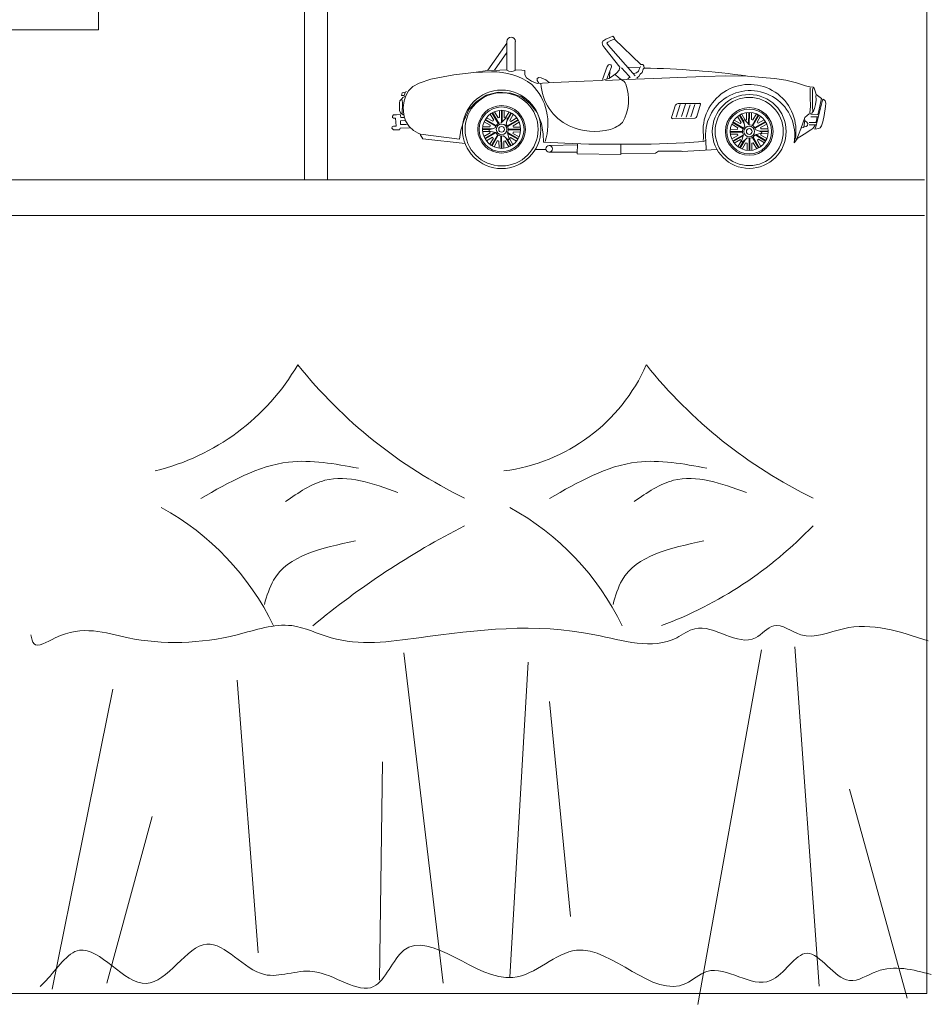
# Model space of a CAD drawing. Units: inches. Extents: x -17 to 1735, y -531 to 60.
# Tile 17 of 27: x 1734.789 to 1734.82808, y -150.26502 to -150.22283. Entities that reach past the tile are written whole.
import ezdxf

# ---------------------------------------------------------------- set-up
doc = ezdxf.new("R2010")
doc.units = ezdxf.units.IN
doc.header["$MEASUREMENT"] = 0
doc.layers.add('A-FURN', color=242, linetype='Continuous', lineweight=18, true_color=0xcd2027)

# ---------------------------------------------------------------- blocks, each defined once
blk = doc.blocks.new('childrens_room_2')
for p, q in [((74.0483, 55.5336), (74.0483, 52.9336)), ((73.1463, 53.9825), (73.1463, 54.7238)), ((73.3706, 53.8193), (73.3706, 54.1771)), ((73.3956, 53.8193), (73.3956, 54.1771)), ((72.0693, 53.9825), (73.1463, 53.9825)), ((73.6988, 53.9726), (73.6953, 53.9704)), ((73.703, 53.9741), (73.6988, 53.9726)), ((73.7062, 53.9758), (73.703, 53.9741)), ((73.7077, 53.9723), (73.7033, 53.9706)), ((73.7071, 53.9751), (73.7062, 53.9758)), ((73.7086, 53.9727), (73.7071, 53.9751)), ((73.7081, 53.9724), (73.7086, 53.9727)), ((73.7368, 53.9448), (73.7081, 53.9724)), ((73.591, 53.9681), (73.5703, 53.9388)), ((73.591, 53.9699), (73.591, 53.9386)), ((73.6001, 53.9382), (73.6001, 53.9699)), ((73.6953, 53.9704), (73.6946, 53.9686)), ((73.6946, 53.9686), (73.6953, 53.9656)), ((73.6953, 53.9656), (73.6975, 53.9626)), ((73.6975, 53.9626), (73.7141, 53.9421)), ((73.7007, 53.9693), (73.6998, 53.968)), ((73.6998, 53.968), (73.7003, 53.9672)), ((73.7003, 53.9672), (73.7041, 53.9626)), ((73.7033, 53.9706), (73.7007, 53.9693)), ((73.7041, 53.9626), (73.7282, 53.9356)), ((73.591, 53.9579), (73.5774, 53.9387)), ((73.7001, 53.9427), (73.6952, 53.9284)), ((73.6998, 53.9292), (73.7047, 53.9422)), ((73.7015, 53.9444), (73.7001, 53.9427)), ((73.7026, 53.945), (73.7015, 53.9444)), ((73.704, 53.9447), (73.7026, 53.945)), ((73.7046, 53.944), (73.704, 53.9447)), ((73.7047, 53.9432), (73.7046, 53.944)), ((73.7047, 53.9422), (73.7047, 53.9432)), ((73.7141, 53.9421), (73.7132, 53.9386)), ((73.7157, 53.9412), (73.7237, 53.9327)), ((73.7356, 53.9413), (73.723, 53.942)), ((73.7342, 53.9377), (73.7354, 53.9405)), ((73.7354, 53.9405), (73.7365, 53.9428)), ((73.7388, 53.9448), (73.7368, 53.9448)), ((73.7402, 53.9433), (73.7388, 53.9448)), ((73.7395, 53.9398), (73.7403, 53.9409)), ((73.7403, 53.9409), (73.7402, 53.9433)), ((73.5333, 53.9338), (73.5083, 53.9288)), ((73.5551, 53.9362), (73.5333, 53.9338)), ((73.57, 53.9382), (73.5551, 53.9362)), ((73.5742, 53.9368), (73.5551, 53.9362)), ((73.5831, 53.9387), (73.57, 53.9382)), ((73.591, 53.9389), (73.5831, 53.9387)), ((73.6073, 53.9386), (73.6001, 53.9389)), ((73.6106, 53.9383), (73.6073, 53.9386)), ((73.6106, 53.9383), (73.6104, 53.9335)), ((73.6104, 53.9335), (73.6123, 53.9305)), ((73.6123, 53.9305), (73.6176, 53.9268)), ((73.6256, 53.9307), (73.6238, 53.9298)), ((73.6238, 53.9298), (73.6238, 53.9275)), ((73.6282, 53.9303), (73.6256, 53.9307)), ((73.6335, 53.9281), (73.6282, 53.9303)), ((73.7019, 53.9297), (73.6944, 53.9276)), ((73.7058, 53.9323), (73.7019, 53.9297)), ((73.7027, 53.9308), (73.703, 53.9372)), ((73.7102, 53.9353), (73.7058, 53.9323)), ((73.7093, 53.9335), (73.7124, 53.9308)), ((73.7132, 53.9386), (73.7102, 53.9353)), ((73.7124, 53.9308), (73.7169, 53.9275)), ((73.751, 53.9297), (73.7208, 53.9284)), ((73.7238, 53.9304), (73.7228, 53.9292)), ((73.7237, 53.9327), (73.7252, 53.9309)), ((73.7252, 53.9309), (73.7238, 53.9304)), ((73.7282, 53.9356), (73.7307, 53.9327)), ((73.7292, 53.935), (73.7319, 53.9358)), ((73.7319, 53.9358), (73.7342, 53.9377)), ((73.7325, 53.93), (73.7335, 53.931)), ((73.7335, 53.931), (73.7345, 53.9319)), ((73.7345, 53.9319), (73.7362, 53.9343)), ((73.7362, 53.9343), (73.7383, 53.9363)), ((73.7383, 53.9363), (73.7395, 53.9398)), ((73.7769, 53.9307), (73.751, 53.9297)), ((73.8064, 53.932), (73.7769, 53.9307)), ((73.8292, 53.9324), (73.8064, 53.932)), ((73.853, 53.9323), (73.8292, 53.9324)), ((73.853, 53.9323), (73.8495, 53.9328)), ((73.8688, 53.9308), (73.853, 53.9323)), ((73.8822, 53.9295), (73.8688, 53.9308)), ((73.8945, 53.9278), (73.8822, 53.9295)), ((73.4884, 53.9208), (73.484, 53.9163)), ((73.4955, 53.9247), (73.4884, 53.9208)), ((73.5083, 53.9288), (73.4955, 53.9247)), ((73.6176, 53.9268), (73.6239, 53.9242)), ((73.6238, 53.9275), (73.6258, 53.9244)), ((73.6416, 53.9252), (73.6239, 53.9242)), ((73.6369, 53.9253), (73.6335, 53.9281)), ((73.6751, 53.9268), (73.6416, 53.9252)), ((73.6944, 53.9276), (73.6751, 53.9268)), ((73.7208, 53.9284), (73.6983, 53.9276)), ((73.9063, 53.9251), (73.8945, 53.9278)), ((73.9161, 53.9218), (73.9063, 53.9251)), ((73.9208, 53.9204), (73.9161, 53.9218)), ((73.9244, 53.9201), (73.9208, 53.9204)), ((73.9212, 53.9195), (73.9213, 53.9094)), ((73.924, 53.919), (73.9237, 53.9167)), ((73.9255, 53.9192), (73.9244, 53.9201)), ((73.9269, 53.9149), (73.9255, 53.9192)), ((73.4764, 53.9111), (73.4768, 53.9141)), ((73.479, 53.9111), (73.4764, 53.9111)), ((73.4766, 53.9075), (73.4778, 53.909)), ((73.4768, 53.9141), (73.4788, 53.9144)), ((73.4778, 53.909), (73.4799, 53.9102)), ((73.4788, 53.9144), (73.4803, 53.9148)), ((73.481, 53.9107), (73.4792, 53.9053)), ((73.4794, 53.9114), (73.4803, 53.9147)), ((73.4803, 53.9148), (73.4818, 53.9155)), ((73.484, 53.9163), (73.481, 53.9107)), ((73.5576, 53.9041), (73.5685, 53.9114)), ((73.5685, 53.9114), (73.5814, 53.9147)), ((73.5814, 53.9147), (73.5954, 53.9137)), ((73.5954, 53.9137), (73.6067, 53.9096)), ((73.6067, 53.9096), (73.6154, 53.9028)), ((73.9213, 53.9094), (73.9215, 53.8992)), ((73.9237, 53.9167), (73.9237, 53.8989)), ((73.9275, 53.9121), (73.9269, 53.9149)), ((73.9273, 53.911), (73.9275, 53.9062)), ((73.9336, 53.9077), (73.9275, 53.9121)), ((73.9329, 53.9045), (73.9336, 53.9079)), ((73.9336, 53.9079), (73.9336, 53.9077)), ((73.474, 53.8949), (73.4742, 53.9033)), ((73.4742, 53.9033), (73.4745, 53.9054)), ((73.4745, 53.9054), (73.4757, 53.9067)), ((73.4757, 53.9067), (73.4766, 53.9075)), ((73.4772, 53.9029), (73.4769, 53.9064)), ((73.4769, 53.8917), (73.4772, 53.9029)), ((73.4792, 53.9053), (73.4779, 53.898)), ((73.4779, 53.898), (73.4787, 53.89)), ((73.5499, 53.8961), (73.5576, 53.9041)), ((73.6154, 53.9028), (73.6239, 53.8928)), ((73.7705, 53.8884), (73.7747, 53.9011)), ((73.7753, 53.8877), (73.7795, 53.9012)), ((73.7782, 53.9025), (73.7986, 53.9024)), ((73.7809, 53.8884), (73.7854, 53.9017)), ((73.786, 53.8875), (73.7904, 53.9009)), ((73.7912, 53.8878), (73.7956, 53.9014)), ((73.8018, 53.9016), (73.7977, 53.8882)), ((73.7986, 53.9024), (73.8009, 53.9026)), ((73.9215, 53.8992), (73.9209, 53.8923)), ((73.9237, 53.8989), (73.924, 53.894)), ((73.9258, 53.897), (73.9248, 53.8942)), ((73.9268, 53.9012), (73.9258, 53.897)), ((73.9275, 53.9062), (73.9268, 53.9012)), ((73.9344, 53.9062), (73.9273, 53.877)), ((73.9309, 53.8964), (73.9329, 53.9045)), ((73.9354, 53.9073), (73.9344, 53.9062)), ((73.9354, 53.9073), (73.9365, 53.9066)), ((73.9377, 53.8991), (73.9363, 53.8894)), ((73.9365, 53.9066), (73.9375, 53.9055)), ((73.9375, 53.9055), (73.9382, 53.9028)), ((73.9382, 53.9028), (73.9377, 53.8991)), ((73.4664, 53.8886), (73.4676, 53.89)), ((73.4666, 53.8873), (73.4664, 53.8886)), ((73.4675, 53.8863), (73.4666, 53.8873)), ((73.4696, 53.8863), (73.4675, 53.8863)), ((73.4676, 53.89), (73.4708, 53.8902)), ((73.4704, 53.8777), (73.4696, 53.8863)), ((73.4708, 53.8902), (73.4746, 53.8905)), ((73.475, 53.8921), (73.474, 53.8949)), ((73.4746, 53.8905), (73.4751, 53.8892)), ((73.4758, 53.8916), (73.475, 53.8921)), ((73.4751, 53.8892), (73.4755, 53.8871)), ((73.4755, 53.8871), (73.4787, 53.8871)), ((73.4778, 53.8905), (73.4758, 53.8916)), ((73.4781, 53.8898), (73.4778, 53.8905)), ((73.4787, 53.89), (73.4804, 53.8836)), ((73.5441, 53.8834), (73.5499, 53.8961)), ((73.5755, 53.8832), (73.5689, 53.887)), ((73.5767, 53.8843), (73.5728, 53.8909)), ((73.5815, 53.8806), (73.5747, 53.8921)), ((73.5822, 53.8809), (73.5753, 53.8925)), ((73.5813, 53.8868), (73.5774, 53.8935)), ((73.5828, 53.8872), (73.5828, 53.8948)), ((73.5851, 53.8816), (73.585, 53.895)), ((73.5852, 53.8816), (73.5901, 53.8869)), ((73.5859, 53.8823), (73.5857, 53.895)), ((73.5881, 53.8871), (73.588, 53.8948)), ((73.5896, 53.8867), (73.5933, 53.8933)), ((73.5901, 53.8869), (73.5915, 53.8863)), ((73.5915, 53.8863), (73.5901, 53.8797)), ((73.5907, 53.8826), (73.596, 53.8919)), ((73.5912, 53.885), (73.5954, 53.8923)), ((73.5941, 53.884), (73.5979, 53.8906)), ((73.5952, 53.8828), (73.6017, 53.8867)), ((73.6239, 53.8928), (73.6285, 53.8805)), ((73.7957, 53.8865), (73.7716, 53.8858)), ((73.8459, 53.8816), (73.8421, 53.8883)), ((73.8493, 53.8802), (73.844, 53.8896)), ((73.8488, 53.8827), (73.8446, 53.89)), ((73.8504, 53.8843), (73.8467, 53.891)), ((73.8519, 53.8848), (73.852, 53.8924)), ((73.8541, 53.8799), (73.8543, 53.8926)), ((73.8549, 53.8792), (73.855, 53.8926)), ((73.8572, 53.8849), (73.8573, 53.8925)), ((73.8579, 53.8786), (73.8647, 53.8902)), ((73.8585, 53.8782), (73.8653, 53.8898)), ((73.8587, 53.8845), (73.8626, 53.8911)), ((73.8633, 53.882), (73.8672, 53.8885)), ((73.9153, 53.8871), (73.9132, 53.8811)), ((73.9179, 53.8893), (73.9153, 53.8871)), ((73.9202, 53.8912), (73.9179, 53.8893)), ((73.9229, 53.892), (73.9202, 53.8912)), ((73.9299, 53.8902), (73.922, 53.8903)), ((73.9295, 53.8878), (73.922, 53.8878)), ((73.9242, 53.8932), (73.9229, 53.892)), ((73.9248, 53.8942), (73.9242, 53.8932)), ((73.9281, 53.8841), (73.9289, 53.8878)), ((73.9295, 53.8902), (73.9309, 53.8964)), ((73.9363, 53.8894), (73.9348, 53.8823)), ((73.4658, 53.8755), (73.466, 53.877)), ((73.466, 53.877), (73.4676, 53.8776)), ((73.4676, 53.8776), (73.4704, 53.8777)), ((73.4849, 53.8758), (73.4749, 53.8755)), ((73.4751, 53.8837), (73.48, 53.8839)), ((73.4752, 53.8796), (73.4751, 53.8837)), ((73.4816, 53.8794), (73.4752, 53.8796)), ((73.4804, 53.8836), (73.4846, 53.8775)), ((73.4846, 53.8775), (73.4894, 53.873)), ((73.5409, 53.8735), (73.5441, 53.8834)), ((73.5724, 53.8772), (73.5647, 53.8771)), ((73.5728, 53.8787), (73.5662, 53.8825)), ((73.5789, 53.8779), (73.5672, 53.8845)), ((73.5793, 53.8785), (73.5676, 53.8851)), ((73.5716, 53.8738), (73.5781, 53.8759)), ((73.5914, 53.878), (73.603, 53.8848)), ((73.5918, 53.8773), (73.6034, 53.8842)), ((73.5977, 53.8782), (73.6043, 53.8821)), ((73.5981, 53.8767), (73.6057, 53.8767)), ((73.6285, 53.8805), (73.6306, 53.8689)), ((73.8423, 53.8759), (73.8357, 53.8798)), ((73.8482, 53.875), (73.8366, 53.8818)), ((73.8486, 53.8757), (73.837, 53.8825)), ((73.8448, 53.8805), (73.8383, 53.8843)), ((73.8499, 53.8846), (73.8485, 53.884)), ((73.8485, 53.884), (73.8499, 53.8773)), ((73.8548, 53.8792), (73.8499, 53.8846)), ((73.8608, 53.8762), (73.8725, 53.8828)), ((73.8612, 53.8755), (73.8728, 53.8821)), ((73.8645, 53.8809), (73.8712, 53.8846)), ((73.8672, 53.8764), (73.8738, 53.8801)), ((73.9132, 53.8811), (73.911, 53.8747)), ((73.9142, 53.8763), (73.912, 53.8758)), ((73.9144, 53.8765), (73.9142, 53.8763)), ((73.9154, 53.8842), (73.9144, 53.8765)), ((73.9167, 53.8773), (73.9145, 53.8771)), ((73.9151, 53.8845), (73.9154, 53.8842)), ((73.9155, 53.8835), (73.917, 53.8826)), ((73.9183, 53.8785), (73.9167, 53.8773)), ((73.917, 53.8826), (73.9185, 53.8808)), ((73.9185, 53.8808), (73.9183, 53.8785)), ((73.9281, 53.8816), (73.9201, 53.8816)), ((73.9277, 53.8792), (73.9201, 53.8792)), ((73.9242, 53.8753), (73.9261, 53.8781)), ((73.9261, 53.8781), (73.9264, 53.8792)), ((73.9273, 53.877), (73.9262, 53.8744)), ((73.9272, 53.8816), (73.9281, 53.8841)), ((73.9322, 53.8761), (73.9306, 53.8751)), ((73.9335, 53.8781), (73.9322, 53.8761)), ((73.9348, 53.8823), (73.9335, 53.8781)), ((73.4676, 53.8737), (73.4658, 53.8755)), ((73.4698, 53.8737), (73.4676, 53.8737)), ((73.4739, 53.8737), (73.4698, 53.8737)), ((73.4749, 53.8755), (73.4739, 53.8737)), ((73.4894, 53.873), (73.4942, 53.8701)), ((73.4942, 53.8701), (73.4969, 53.8692)), ((73.4995, 53.8641), (73.4965, 53.8688)), ((73.4969, 53.8692), (73.5392, 53.8636)), ((73.5392, 53.8636), (73.5409, 53.8735)), ((73.5752, 53.875), (73.5645, 53.8749)), ((73.5729, 53.8742), (73.5645, 53.8741)), ((73.5723, 53.872), (73.5646, 53.8719)), ((73.5727, 53.8704), (73.566, 53.8665)), ((73.5779, 53.8709), (73.567, 53.8645)), ((73.5789, 53.8706), (73.5674, 53.8638)), ((73.5752, 53.8658), (73.5686, 53.8619)), ((73.5718, 53.8723), (73.5716, 53.8738)), ((73.5789, 53.8707), (73.5718, 53.8723)), ((73.581, 53.8684), (73.5743, 53.8567)), ((73.5816, 53.868), (73.575, 53.8563)), ((73.5845, 53.8671), (73.5846, 53.8536)), ((73.5852, 53.867), (73.5854, 53.8536)), ((73.5924, 53.8628), (73.5873, 53.8674)), ((73.5896, 53.8654), (73.595, 53.8561)), ((73.5915, 53.8707), (73.6032, 53.8641)), ((73.5915, 53.8706), (73.5936, 53.8637)), ((73.5917, 53.8697), (73.6028, 53.8635)), ((73.5924, 53.8736), (73.6059, 53.8737)), ((73.5925, 53.8744), (73.6059, 53.8745)), ((73.5948, 53.8654), (73.6015, 53.8616)), ((73.5975, 53.8699), (73.6042, 53.8662)), ((73.598, 53.8714), (73.6057, 53.8715)), ((73.6306, 53.8689), (73.631, 53.8603)), ((73.8045, 53.8741), (73.8051, 53.8651)), ((73.8051, 53.8651), (73.8048, 53.8622)), ((73.8476, 53.8713), (73.8341, 53.8714)), ((73.8476, 53.872), (73.8342, 53.8721)), ((73.8419, 53.8743), (73.8343, 53.8744)), ((73.842, 53.8691), (73.8343, 53.8691)), ((73.8425, 53.8676), (73.8358, 53.8638)), ((73.8485, 53.8684), (73.8368, 53.8618)), ((73.8483, 53.8674), (73.8372, 53.8611)), ((73.8485, 53.8683), (73.8464, 53.8613)), ((73.8476, 53.8605), (73.8527, 53.865)), ((73.8584, 53.8656), (73.865, 53.854)), ((73.859, 53.866), (73.8657, 53.8543)), ((73.8611, 53.8684), (73.8682, 53.87)), ((73.8611, 53.8683), (73.8726, 53.8615)), ((73.8684, 53.8714), (73.8619, 53.8736)), ((73.8621, 53.8686), (73.873, 53.8621)), ((73.8648, 53.8726), (73.8755, 53.8725)), ((73.8671, 53.8719), (73.8755, 53.8718)), ((73.8674, 53.8681), (73.874, 53.8642)), ((73.8676, 53.8748), (73.8753, 53.8748)), ((73.8677, 53.8696), (73.8754, 53.8695)), ((73.8682, 53.87), (73.8684, 53.8714)), ((73.9085, 53.8682), (73.9057, 53.862)), ((73.9071, 53.8645), (73.9147, 53.8689)), ((73.911, 53.8747), (73.9085, 53.8682)), ((73.9147, 53.8689), (73.9219, 53.8736)), ((73.9219, 53.8736), (73.9242, 53.8753)), ((73.9306, 53.8751), (73.9262, 53.8744)), ((73.5455, 53.859), (73.4995, 53.8641)), ((73.5763, 53.8647), (73.5725, 53.858)), ((73.5808, 53.862), (73.577, 53.8553)), ((73.5823, 53.8615), (73.5824, 53.8538)), ((73.5875, 53.8614), (73.5876, 53.8538)), ((73.5891, 53.8618), (73.593, 53.8552)), ((73.5914, 53.8637), (73.5957, 53.8565)), ((73.5936, 53.8637), (73.5924, 53.8628)), ((73.5937, 53.8643), (73.5975, 53.8577)), ((73.631, 53.8603), (73.6542, 53.8593)), ((73.6369, 53.8567), (73.6678, 53.8573)), ((73.6542, 53.8593), (73.68, 53.8583)), ((73.6676, 53.8477), (73.668, 53.8586)), ((73.68, 53.8583), (73.7124, 53.858)), ((73.7124, 53.858), (73.7479, 53.8581)), ((73.7149, 53.8579), (73.7149, 53.8469)), ((73.7845, 53.8598), (73.7479, 53.8581)), ((73.7845, 53.8598), (73.8046, 53.8611)), ((73.8046, 53.8611), (73.8076, 53.8622)), ((73.8076, 53.8622), (73.8081, 53.8517)), ((73.8452, 53.8631), (73.8385, 53.8593)), ((73.8463, 53.862), (73.8425, 53.8554)), ((73.8486, 53.8614), (73.8443, 53.8541)), ((73.8504, 53.863), (73.845, 53.8538)), ((73.8464, 53.8613), (73.8476, 53.8605)), ((73.8509, 53.8594), (73.847, 53.8528)), ((73.8525, 53.8591), (73.8524, 53.8514)), ((73.8548, 53.8647), (73.8546, 53.8513)), ((73.8555, 53.8647), (73.8554, 53.8513)), ((73.8577, 53.8592), (73.8576, 53.8515)), ((73.8592, 53.8596), (73.863, 53.853)), ((73.8637, 53.8623), (73.8675, 53.8556)), ((73.8648, 53.8635), (73.8714, 53.8596)), ((73.9038, 53.8597), (73.9053, 53.8613)), ((73.9053, 53.8613), (73.9069, 53.8641)), ((73.9069, 53.8641), (73.9071, 53.8645)), ((73.6333, 53.8524), (73.6223, 53.8524)), ((73.6678, 53.8495), (73.6368, 53.8495)), ((73.7149, 53.8469), (73.6676, 53.8477)), ((73.7528, 53.8483), (73.7149, 53.8479)), ((73.7562, 53.8507), (73.7528, 53.8483)), ((73.7811, 53.8506), (73.7562, 53.8507)), ((73.7819, 53.8503), (73.7811, 53.8506)), ((73.7819, 53.8503), (73.8197, 53.8523)), ((73.0463, 53.8193), (74.0458, 53.8193)), ((73.0463, 53.7804), (74.0458, 53.7804)), ((73.8682, 53.3077), (73.7989, 52.9219)), ((73.9045, 53.311), (73.9309, 52.9417)), ((73.4788, 53.3044), (73.5217, 52.945)), ((73.6141, 53.2945), (73.5943, 52.9516)), ((73.1619, 53.2648), (73.0959, 52.9384)), ((73.2972, 53.2747), (73.3203, 52.978)), ((73.6372, 53.2516), (73.6603, 53.0175)), ((73.4557, 53.1857), (73.4524, 52.9483)), ((73.9639, 53.156), (74.0266, 52.9285)), ((73.2048, 53.1263), (73.1553, 52.945)), ((72.0483, 52.9336), (74.0483, 52.9336))]:
    blk.add_line(p, q)
blk.add_lwpolyline([(73.628, 53.9242, 0.277279), (73.6587, 53.8781, 0.17984), (73.7036, 53.8743, 0.128199), (73.7167, 53.8819, 0.227122), (73.7203, 53.9236, 0.200085), (73.7159, 53.9282, 1.871987)], format="xyb")
for centre, radius in [((73.5852, 53.8743), 0.0427), ((73.5852, 53.8743), 0.0398), ((73.8548, 53.872), 0.0402), ((73.8548, 53.872), 0.0371), ((73.5852, 53.8743), 0.0259), ((73.5852, 53.8743), 0.0244), ((73.8548, 53.872), 0.0259), ((73.5852, 53.8743), 0.0207), ((73.8548, 53.872), 0.0244), ((73.8548, 53.872), 0.0207), ((73.5852, 53.8743), 0.00582), ((73.5852, 53.8743), 0.00313), ((73.8548, 53.872), 0.00582), ((73.8548, 53.872), 0.00313), ((73.6369, 53.8531), 0.00358)]:
    blk.add_circle(centre, radius)
for centre, radius, start, end in [((73.5956, 53.9699), 0.00456, 0, 180), ((73.725, 52.9996), 0.9415, 82.1883, 89.069), ((73.5773, 53.8693), 0.0675, 52.7792, 92.6699), ((73.5959, 53.9473), 0.01, 240.6981, 294.7246), ((73.5751, 53.8805), 0.0606, 341.2239, 44.7052), ((73.8551, 53.8726), 0.0506, 349.8147, 178.3468), ((73.8558, 53.8679), 0.0486, 350.3249, 186.7561), ((73.7778, 53.8985), 0.00399, 83.8396, 139.4858), ((73.8008, 53.9016), 0.00104, 1.1933, 81.4781), ((73.5852, 53.8743), 0.0131, 100.363, 107.2977), ((73.5852, 53.8743), 0.0131, 70.363, 77.2977), ((73.772, 53.8875), 0.00178, 149.6689, 255.8381), ((73.7942, 53.8902), 0.00408, 292.5869, 329.881), ((73.5852, 53.8743), 0.0131, 160.363, 167.2977), ((73.5852, 53.8743), 0.0131, 130.363, 137.2977), ((73.5852, 53.8743), 0.00727, 89.6688, 167.3416), ((73.5852, 53.8743), 0.00727, 329.6688, 47.3416), ((73.5852, 53.8743), 0.0131, 40.363, 47.2977), ((73.5852, 53.8743), 0.0131, 10.363, 17.2977), ((73.8548, 53.872), 0.0131, 162.7023, 169.637), ((73.8548, 53.872), 0.0131, 132.7023, 139.637), ((73.8548, 53.872), 0.00727, 132.6584, 210.3312), ((73.8548, 53.872), 0.0131, 102.7023, 109.637), ((73.8548, 53.872), 0.00727, 12.6584, 90.3312), ((73.8548, 53.872), 0.0131, 72.7023, 79.637), ((73.8548, 53.872), 0.0131, 42.7023, 49.637), ((73.8548, 53.872), 0.0131, 12.7023, 19.637), ((73.5852, 53.8743), 0.0131, 190.363, 197.2977), ((73.5852, 53.8743), 0.0131, 220.363, 227.2977), ((73.5852, 53.8743), 0.00727, 209.6688, 287.3416), ((73.5852, 53.8743), 0.0131, 310.363, 317.2977), ((73.5852, 53.8743), 0.0131, 340.363, 347.2977), ((73.8548, 53.872), 0.0131, 192.7023, 199.637), ((73.8548, 53.872), 0.00727, 252.6584, 330.3312), ((73.8548, 53.872), 0.0131, 342.7023, 349.637), ((73.5852, 53.8743), 0.0131, 250.363, 257.2977), ((73.5852, 53.8743), 0.0131, 280.363, 287.2977), ((73.8548, 53.872), 0.0131, 222.7023, 229.637), ((73.8548, 53.872), 0.0131, 252.7023, 259.637), ((73.8548, 53.872), 0.0131, 282.7023, 289.637), ((73.8548, 53.872), 0.0131, 312.7023, 319.637), ((73.1502, 53.7424), 0.2467, 283.5813, 329.71), ((73.7772, 53.9498), 0.5305, 218.7196, 244.019), ((73.5631, 53.6975), 0.1965, 277.1803, 336.111), ((74.1567, 53.9498), 0.5305, 218.7196, 244.019), ((73.0758, 53.2084), 0.2897, 25.7037, 61.3417), ((73.4553, 53.2084), 0.2897, 25.7037, 61.3417), ((73.9661, 52.6242), 0.9207, 117.2353, 129.5593), ((73.6052, 53.7473), 0.441, 290.4483, 316.3463)]:
    blk.add_arc(centre, radius, start, end)
for points, knots in [([(73.4293, 53.5055), (73.4036, 53.5102), (73.343, 53.5214), (73.2888, 53.4904), (73.2576, 53.4725)], [0, 0, 0, 0, 0.0761966, 0.1797644, 0.1797644, 0.1797644, 0.1797644]), ([(73.8088, 53.5055), (73.7831, 53.5102), (73.7225, 53.5214), (73.6684, 53.4904), (73.6372, 53.4725)], [0, 0, 0, 0, 0.0761966, 0.1797644, 0.1797644, 0.1797644, 0.1797644]), ([(73.4722, 53.4791), (73.4449, 53.4888), (73.401, 53.5044), (73.364, 53.4789), (73.3501, 53.4692)], [0, 0, 0, 0, 0.0803017, 0.1290207, 0.1290207, 0.1290207, 0.1290207]), ([(73.8517, 53.4791), (73.8244, 53.4888), (73.7806, 53.5044), (73.7436, 53.4789), (73.7296, 53.4692)], [0, 0, 0, 0, 0.0803017, 0.1290207, 0.1290207, 0.1290207, 0.1290207]), ([(73.3269, 53.3571), (73.3297, 53.3665), (73.342, 53.4085), (73.3892, 53.4185), (73.426, 53.4264)], [0, 0, 0, 0, 0.0281737, 0.1270574, 0.1270574, 0.1270574, 0.1270574]), ([(73.7065, 53.3571), (73.7092, 53.3665), (73.7215, 53.4085), (73.7688, 53.4185), (73.8055, 53.4264)], [0, 0, 0, 0, 0.0281737, 0.1270574, 0.1270574, 0.1270574, 0.1270574]), ([(74.0497, 53.3176), (74.0189, 53.3277), (73.9727, 53.3429), (73.9162, 53.3142), (73.8826, 53.3429), (73.8515, 53.302), (73.8078, 53.3439), (73.757, 53.3046), (73.6493, 53.3411), (73.5288, 53.3257), (73.415, 53.3098), (73.3522, 53.3419), (73.2782, 53.3149), (73.1889, 53.3122), (73.1223, 53.3382), (73.076, 53.307), (73.0736, 53.3202), (73.0728, 53.3242)], [0, 0, 0, 0, 0.0933489, 0.1400233, 0.1713311, 0.1951231, 0.2618688, 0.284004, 0.373177, 0.5646307, 0.660344, 0.7052307, 0.765456, 0.8843182, 0.9635283, 0.9875541, 0.9979816, 0.9979816, 0.9979816, 0.9979816]), ([(74.053, 52.9544), (74.033, 52.9597), (74.0024, 52.9677), (73.9559, 52.934), (73.9182, 53.003), (73.8761, 52.9212), (73.8199, 52.9738), (73.7593, 52.9152), (73.6784, 53.0196), (73.5881, 52.9128), (73.4862, 53.0274), (73.4479, 52.9163), (73.3839, 52.972), (73.32, 52.9378), (73.261, 53.0217), (73.2001, 52.9041), (73.1314, 53.0091), (73.0987, 52.9567), (73.0849, 52.9434), (73.0827, 52.9412)], [0, 0, 0, 0, 0.059499, 0.090806, 0.145719, 0.195208, 0.265218, 0.291821, 0.416049, 0.491443, 0.613907, 0.665431, 0.733467, 0.786377, 0.857224, 0.935928, 1.01709, 1.066132, 1.075462, 1.075462, 1.075462, 1.075462])]:
    blk.add_open_spline(points, degree=3, knots=knots)

msp = doc.modelspace()

# ---------------------------------------------------------------- block references
at = {"layer": 'A-FURN', "xscale": 0.0393700787401575, "yscale": 0.0393700787401575, "zscale": 0.0393700787401575}
msp.add_blockref('childrens_room_2', (1731.912601, -152.348565), dxfattribs=at)

doc.saveas('drawing.dxf')
